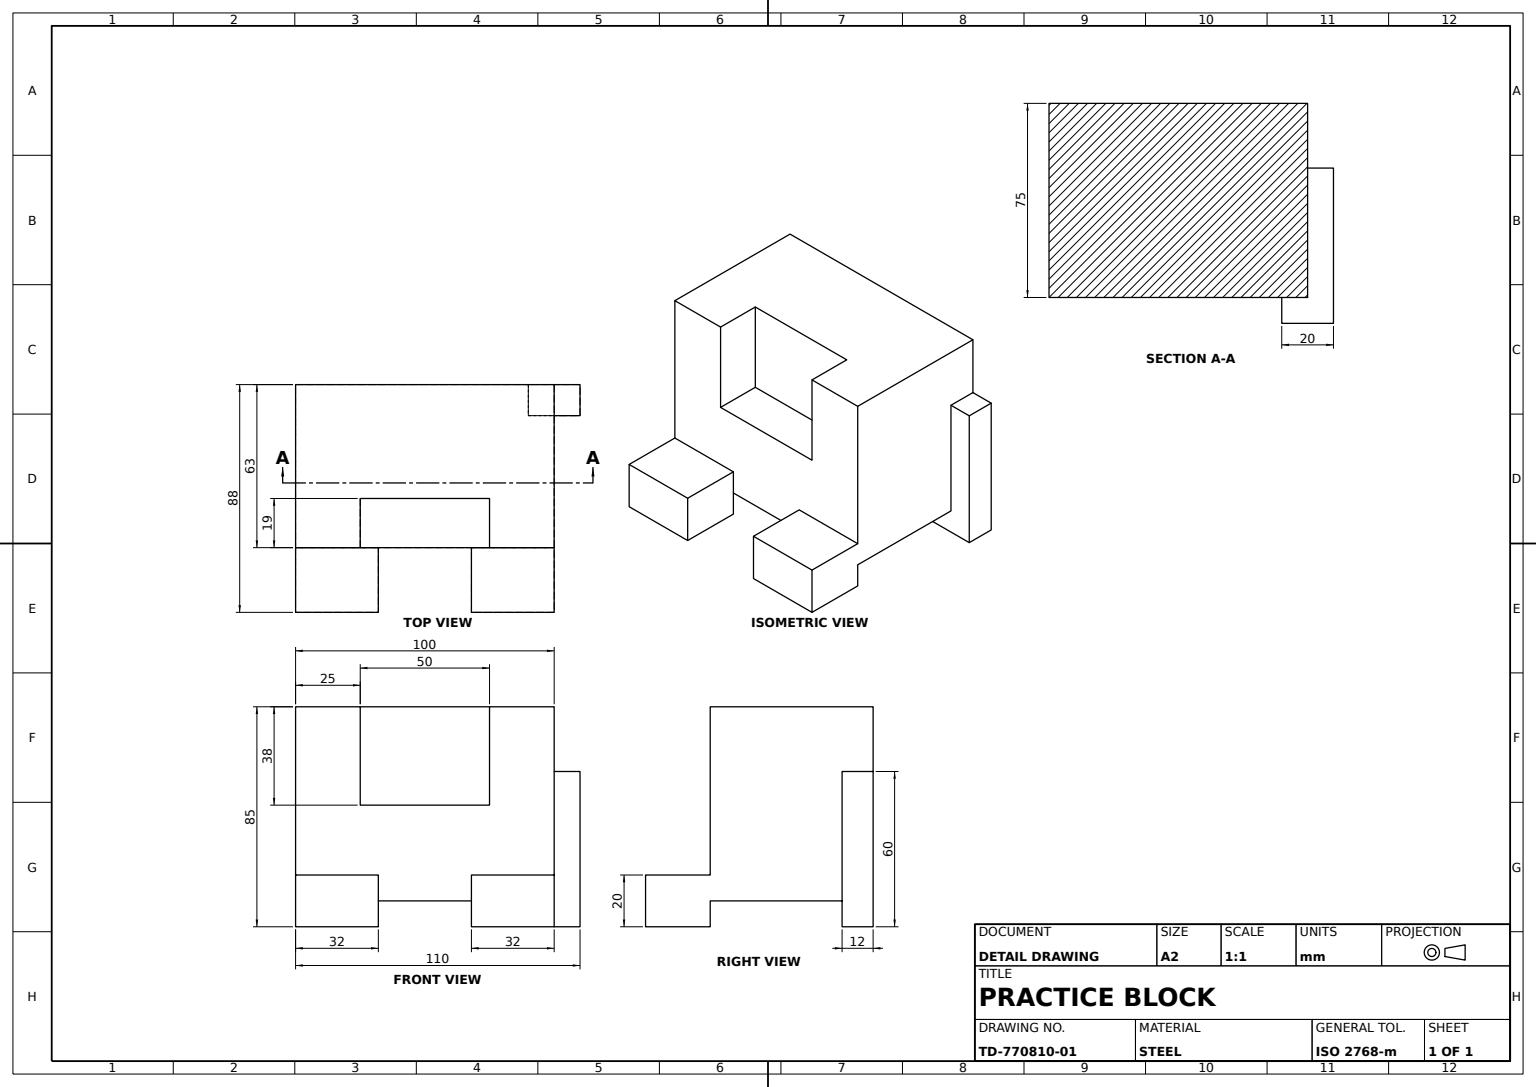
SolidWorks part; units mm, degrees
material "Plain Carbon Steel"
ref_plane "Front Plane" through (0, 0, 0) normal (0, 0, 1) x (1, 0, 0)
ref_plane "Top Plane" through (0, 0, 0) normal (0, 1, 0) x (1, 0, 0)
ref_plane "Right Plane" through (0, 0, 0) normal (1, 0, 0) x (0, 0, -1)
sketch "Base Block Sketch" plane through (0, 0, 0) normal (0, 1, 0) x (1, 0, 0)
  line L0 (0, 0) -> (0, 63)
  line L1 (0, 63) -> (100, 63)
  line L2 (100, 63) -> (100, 0)
  line L3 (100, 0) -> (0, 0)
  dimension "D1" = 100
  dimension "D2" = 63
extrude "Base Block 100x63x75" add sketch "Base Block Sketch" along normal blind 75
sketch "Top Pocket Sketch" plane through (0, 0, 0) normal (0, 0, 1) x (1, 0, 0)
  line L0 (25, 75) -> (25, 37)
  line L1 (0, 75) -> (100, 75) construction
  line L2 (25, 37) -> (75, 37)
  line L3 (75, 37) -> (75, 75)
  line L4 (75, 75) -> (25, 75)
  line L5 (100, 75) -> (100, 0) construction
  dimension "D1" = 38
  dimension "D2" = 25
  dimension "D3" = 25
extrude "Top Pocket 38x25x19" cut sketch "Top Pocket Sketch" against normal blind 19
sketch "Feet Sketch" plane through (0, 0, 0) normal (0, -1, 0) x (1, 0, 0)
  line L0 (0, 0) -> (0, 25)
  line L1 (0, 25) -> (32, 25)
  line L2 (32, 25) -> (32, 0)
  line L3 (0, 0) -> (100, 0) construction
  line L4 (32, 0) -> (0, 0)
  line L5 (100, 0) -> (100, 25)
  line L6 (100, 25) -> (68, 25)
  line L7 (68, 25) -> (68, 0)
  line L8 (68, 0) -> (100, 0)
  dimension "D1" = 32
  dimension "D2" = 25
  dimension "D3" = 32
  dimension "D4" = 25
extrude "Feet 2x 32x25" add sketch "Feet Sketch" along normal mid plane 20
sketch "Side Rib Sketch" plane through (100, 0, 0) normal (1, 0, 0) x (0, 0, -1)
  line L0 (63, 0) -> (63, 50)
  line L1 (63, 75) -> (63, 0) construction
  line L2 (63, 50) -> (51, 50)
  line L6 (51, 50) -> (51, -10)
  line L7 (51, -10) -> (63, -10)
  line L8 (63, -10) -> (63, 0)
  dimension "D1" = 60
  dimension "D2" = 50
  dimension "D3" = 12
extrude "Side Rib" add sketch "Side Rib Sketch" along normal mid plane 20
